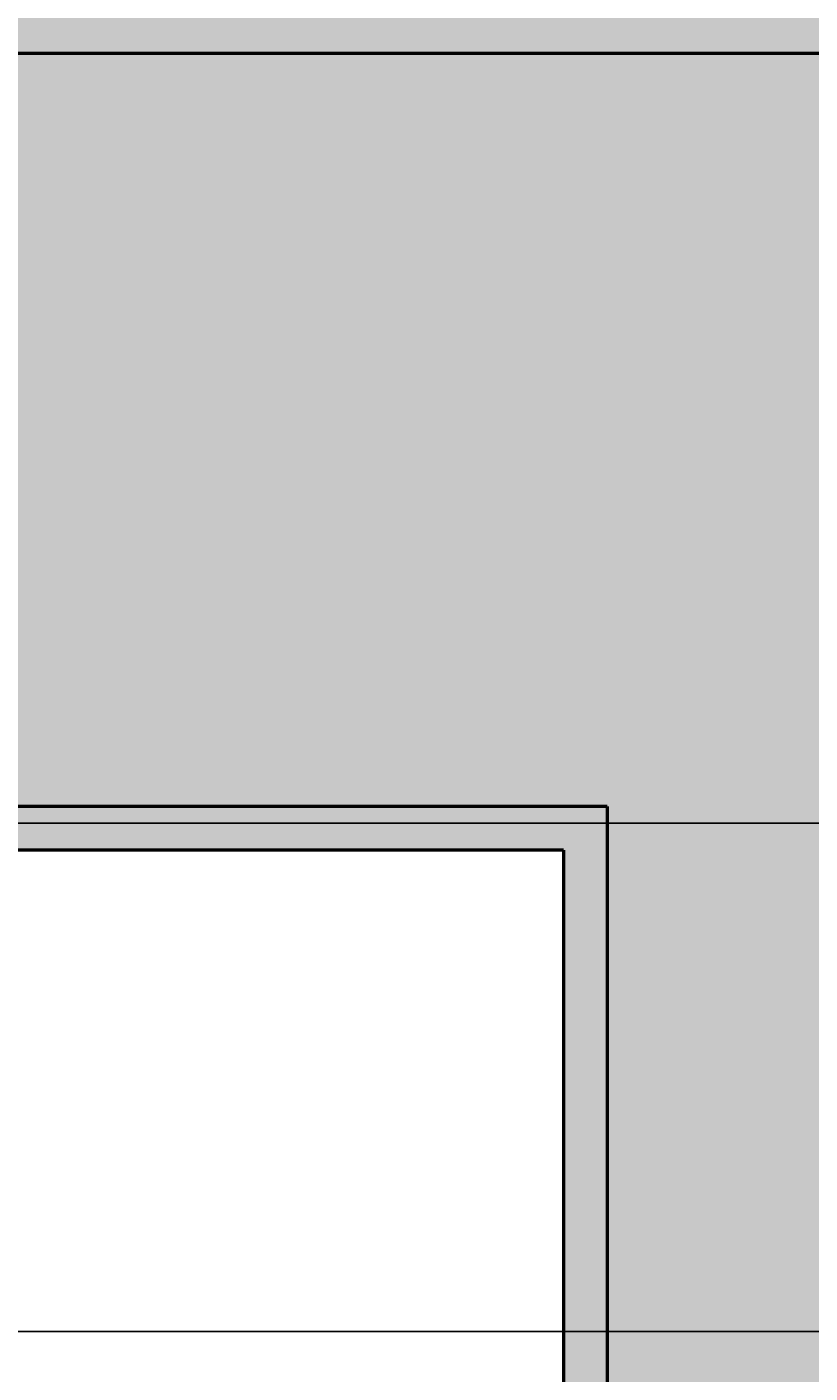
# Model space of a CAD drawing. Units: inches. Extents: x -12 to 334, y -10 to 186.
# Tile 5 of 77: x 24 to 42, y 49 to 79. Entities that reach past the tile are written whole.
import ezdxf

# ---------------------------------------------------------------- set-up
doc = ezdxf.new("R2010")
doc.units = ezdxf.units.IN
doc.header["$MEASUREMENT"] = 0
for name, color, linetype, lineweight in [('M-DIMS', 2, 'Continuous', 18), ('M-EQPM', 7, 'Continuous', 50), ('M-EQPM-PATT', 8, 'Continuous', 18)]:
    doc.layers.add(name, color=color, linetype=linetype, lineweight=lineweight)
doc.styles.get("Standard").update_dxf_attribs({"font": 'arial.ttf'})
doc.dimstyles.get("Standard").update_dxf_attribs({"dimtxt": 0.18, "dimasz": 0.18, "dimexe": 0.18, "dimexo": 0.0625, "dimgap": 0.09, "dimtad": 0, "dimtih": 1, "dimtoh": 1, "dimdec": 4, "dimzin": 0, "dimdsep": 46, "dimtxsty": 'Standard', "dimcen": 0.09, "dimadec": 0, "dimazin": 0, "dimtfac": 1, "dimtdec": 4, "dimtofl": 0, "dimtmove": 0, "dimatfit": 3, "dimfxl": 1, "dimtolj": 1, "dimtzin": 0, "dimarcsym": 0})

# ---------------------------------------------------------------- blocks, each defined once
blk = doc.blocks.new('*D1')
at = {"layer": 'Defpoints', "color": 0, "transparency": 16777216}
for p in [(281.426, 91.899), (3.376, 80.692), (281.426, 14.304)]:
    blk.add_point(p, dxfattribs=at)
at = {"layer": 'M-DIMS', "color": 0, "lineweight": -2, "transparency": 16777216}
for p, q in [((281.426, 91.836), (281.426, 14.124)), ((3.376, 80.629), (3.376, 14.124)), ((3.556, 14.304), (141.935, 14.304)), ((281.246, 14.304), (142.867, 14.304))]:
    blk.add_line(p, q, dxfattribs=at)
at = {"layer": 'M-DIMS', "color": 0, "transparency": 16777216}
for points in [[(3.556, 14.334), (3.556, 14.274), (3.376, 14.304)], [(281.246, 14.334), (281.246, 14.274), (281.426, 14.304)]]:
    blk.add_solid(points, dxfattribs=at)
at = {"layer": 'M-DIMS', "color": 0, "transparency": 16777216, "insert": (142.401, 14.304), "char_height": 0.18, "attachment_point": 5}
blk.add_mtext('\\A1;278.05', dxfattribs=at)
blk = doc.blocks.new('*D6')
at = {"layer": 'Defpoints', "color": 0, "transparency": 16777216}
for p in [(-11.174, 60.487), (23.581, 60.487), (32.1, 33.675)]:
    blk.add_point(p, dxfattribs=at)
at = {"layer": 'M-DIMS', "color": 0, "lineweight": -2, "transparency": 16777216}
for p, q in [((23.518, 60.487), (-11.354, 60.487)), ((-11.174, 60.307), (-11.174, 47.263)), ((-11.174, 33.855), (-11.174, 46.899)), ((32.038, 33.675), (-11.354, 33.675))]:
    blk.add_line(p, q, dxfattribs=at)
at = {"layer": 'M-DIMS', "color": 0, "transparency": 16777216}
for points in [[(-11.204, 60.307), (-11.144, 60.307), (-11.174, 60.487)], [(-11.204, 33.855), (-11.144, 33.855), (-11.174, 33.675)]]:
    blk.add_solid(points, dxfattribs=at)
at = {"layer": 'M-DIMS', "color": 0, "transparency": 16777216, "insert": (-11.174, 47.081), "char_height": 0.18, "attachment_point": 5}
blk.add_mtext('\\A1;26.81', dxfattribs=at)
blk = doc.blocks.new('*D14')
at = {"layer": 'Defpoints', "color": 0, "transparency": 16777216}
for p in [(63.5, 109.058), (-11.174, 49.45), (64.207, 49.45)]:
    blk.add_point(p, dxfattribs=at)
at = {"layer": 'M-DIMS', "color": 0, "lineweight": -2, "transparency": 16777216}
for p, q in [((63.438, 109.058), (-11.354, 109.058)), ((-11.174, 108.878), (-11.174, 79.436)), ((-11.174, 49.63), (-11.174, 79.072)), ((64.144, 49.45), (-11.354, 49.45))]:
    blk.add_line(p, q, dxfattribs=at)
at = {"layer": 'M-DIMS', "color": 0, "transparency": 16777216}
for points in [[(-11.204, 108.878), (-11.144, 108.878), (-11.174, 109.058)], [(-11.204, 49.63), (-11.144, 49.63), (-11.174, 49.45)]]:
    blk.add_solid(points, dxfattribs=at)
at = {"layer": 'M-DIMS', "color": 0, "transparency": 16777216, "insert": (-11.174, 79.254), "char_height": 0.18, "attachment_point": 5}
blk.add_mtext('\\A1;59.61', dxfattribs=at)
blk = doc.blocks.new('*D35')
at = {"layer": 'Defpoints', "color": 0, "transparency": 16777216}
for p in [(216.428, 98.108), (-11.174, 61.105), (216.428, 61.105)]:
    blk.add_point(p, dxfattribs=at)
at = {"layer": 'M-DIMS', "color": 0, "lineweight": -2, "transparency": 16777216}
for p, q in [((216.365, 98.108), (-11.354, 98.108)), ((-11.174, 97.928), (-11.174, 79.788)), ((-11.174, 61.285), (-11.174, 79.424)), ((216.365, 61.105), (-11.354, 61.105))]:
    blk.add_line(p, q, dxfattribs=at)
at = {"layer": 'M-DIMS', "color": 0, "transparency": 16777216}
for points in [[(-11.204, 97.928), (-11.144, 97.928), (-11.174, 98.108)], [(-11.204, 61.285), (-11.144, 61.285), (-11.174, 61.105)]]:
    blk.add_solid(points, dxfattribs=at)
at = {"layer": 'M-DIMS', "color": 0, "transparency": 16777216, "insert": (-11.174, 79.606), "char_height": 0.18, "attachment_point": 5}
blk.add_mtext('\\A1;37', dxfattribs=at)
blk = doc.blocks.new('*D39')
at = {"layer": 'Defpoints', "color": 0, "transparency": 16777216}
for p in [(279.726, 80.692), (-11.174, 45.854), (269.381, 45.854)]:
    blk.add_point(p, dxfattribs=at)
at = {"layer": 'M-DIMS', "color": 0, "lineweight": -2, "transparency": 16777216}
for p, q in [((279.664, 80.692), (-11.354, 80.692)), ((-11.174, 80.512), (-11.174, 63.455)), ((-11.174, 46.034), (-11.174, 63.091)), ((269.318, 45.854), (-11.354, 45.854))]:
    blk.add_line(p, q, dxfattribs=at)
at = {"layer": 'M-DIMS', "color": 0, "transparency": 16777216}
for points in [[(-11.204, 80.512), (-11.144, 80.512), (-11.174, 80.692)], [(-11.204, 46.034), (-11.144, 46.034), (-11.174, 45.854)]]:
    blk.add_solid(points, dxfattribs=at)
at = {"layer": 'M-DIMS', "color": 0, "transparency": 16777216, "insert": (-11.174, 63.273), "char_height": 0.18, "attachment_point": 5}
blk.add_mtext('\\A1;34.84', dxfattribs=at)

msp = doc.modelspace()

# ---------------------------------------------------------------- hatches: boundary and pattern name
at = {"layer": 'M-EQPM-PATT'}
h = msp.add_hatch(color=256, dxfattribs=at)
h.set_gradient(color1=(99, 100, 102), color2=(99, 100, 102), tint=1)
h.paths.add_polyline_path([(4.3766, 80.754, -0.4132606), (23.5807, 99.8958), (37.1002, 99.8958), (37.1002, 127.7078), (32.1002, 127.7078), (32.1002, 125.2078), (36.1002, 125.2078), (36.1002, 100.8958), (23.5807, 100.8958, 1), (23.5807, 60.4872), (36.1002, 60.4872), (36.1002, 36.1752), (32.1002, 36.1752), (32.1002, 33.6752), (37.1002, 33.6752), (37.1002, 61.4872), (23.5807, 61.4872, -0.384914), (4.4744, 78.754), (72.9244, 78.754), (72.9244, 69.6117), (75.9244, 69.6117), (75.9244, 89.8963), (72.9244, 89.8963), (72.9244, 80.754)])
h.paths.add_polyline_path([(54.1002, 125.2078), (58.1002, 125.2078), (58.1002, 127.7078), (53.1002, 127.7078), (53.1002, 99.8958), (64.5, 99.8958), (64.5, 109.0583), (63.5, 109.0583), (63.5, 100.8958), (54.1002, 100.8958)], flags=17)
h.paths.add_polyline_path([(53.1002, 33.6752), (58.1002, 33.6752), (58.1002, 36.1752), (54.1002, 36.1752), (54.1002, 60.4872), (64.2068, 60.4872), (64.2068, 49.4497), (87.8879, 49.4497), (87.8879, 55.3205), (104.8919, 55.3205), (104.8919, 30.8541), (99.8919, 30.8541), (99.8919, 28.8541), (105.8919, 28.8541), (105.8919, 56.3205), (87.8879, 56.3205), (87.8879, 63.6117), (86.8879, 63.6117), (86.8879, 50.4497), (65.0061, 50.4497), (65.0061, 63.6117), (64.5, 63.6117), (64.5, 61.4872), (53.1002, 61.4872)])
h.paths.add_polyline_path([(121.8919, 28.8541), (121.8919, 30.8541), (116.8919, 30.8541), (116.8919, 45.8541), (209.6965, 45.8541), (209.9204, 46.8541), (115.8919, 46.8541), (115.8919, 28.8541)])
h.paths.add_polyline_path([(221.5761, 32.8541), (216.5761, 32.8541), (216.5761, 30.8541), (222.5761, 30.8541), (222.5761, 46.8541), (209.9204, 46.8541), (209.6965, 45.8541), (221.5761, 45.8541)])
h.paths.add_polyline_path([(233.5761, 45.8541), (249.8485, 45.8541), (249.3759, 46.8541), (232.5761, 46.8541), (232.5761, 30.8541), (238.5761, 30.8541), (238.5761, 32.8541), (233.5761, 32.8541)])
h = msp.add_hatch(color=256, dxfattribs=at)
h.set_gradient(color1=(205, 32, 39), color2=(205, 32, 39), tint=1)
h.paths.add_polyline_path([(64.5, 80.754), (64.5, 89.8963), (226.6083, 89.8963, -1), (226.6083, 69.6117), (64.5, 69.6117), (64.5, 78.754), (4.4744, 78.754, 0.384914), (23.5807, 61.4872), (37.1002, 61.4872), (37.1002, 33.6752), (53.1002, 33.6752), (53.1002, 61.4872), (64.5, 61.4872), (64.5, 63.6117), (226.6083, 63.6117, 1), (226.6083, 95.8963), (64.5, 95.8963), (64.5, 99.8958), (53.1002, 99.8958), (53.1002, 127.7078), (37.1002, 127.7078), (37.1002, 99.8958), (23.5807, 99.8958, 0.4132606), (4.3766, 80.754)])
h.paths.add_polyline_path([(64.5, 91.8963), (64.5, 93.8963), (226.6083, 93.8963, -1), (226.6083, 65.6117), (64.5, 65.6117), (64.5, 67.6117), (226.6083, 67.6117, 1), (226.6083, 91.8963)], flags=16)

# ---------------------------------------------------------------- linework, layer by layer
at = {"layer": 'M-EQPM'}
for p, q in [((72.9244, 78.754), (4.4744, 78.754)), ((37.1002, 61.4872), (37.1002, 33.6752)), ((36.1002, 60.4872), (36.1002, 36.1752))]:
    msp.add_line(p, q, dxfattribs=at)
for points in [[(36.1002, 60.4872), (23.5807, 60.4872, -1), (23.5807, 100.8958), (36.1002, 100.8958)], [(37.1002, 61.4872), (23.5807, 61.4872, -0.384914), (4.4744, 78.754, -0.384914)]]:
    msp.add_lwpolyline(points, format="xyb", dxfattribs=at)

# ---------------------------------------------------------------- dimensions: what is measured, and where the dimension line sits
at = {"layer": 'M-DIMS'}
for base, p1, p2, override, picture, middle in [((-11.1736, 49.4497), (63.5, 109.0583), (64.2068, 49.4497), {"dimdec": 2, "dimlfac": 1, "dimrnd": 0, "dimzin": 0, "dimdsep": 46, "dimlunit": 2}, '*D14', (-11.1735, 79.254)), ((-11.1736, 61.1045), (216.4278, 98.1081), (216.4278, 61.1045), {"dimdec": 0, "dimlfac": 1, "dimrnd": 0, "dimzin": 0, "dimdsep": 46, "dimlunit": 2}, '*D35', (-11.1735, 79.6063)), ((-11.1736, 45.8541), (279.7263, 80.6915), (269.3808, 45.8541), {"dimdec": 2, "dimlfac": 1, "dimrnd": 0, "dimzin": 0, "dimdsep": 46, "dimlunit": 2}, '*D39', (-11.1735, 63.2728)), ((-11.1736, 60.4872), (32.1002, 33.6752), (23.5807, 60.4872), {"dimdec": 2, "dimlfac": 1, "dimrnd": 0, "dimzin": 0, "dimdsep": 46, "dimlunit": 2}, '*D6', (-11.1735, 47.0812))]:
    dim = msp.add_linear_dim(base=base, p1=p1, p2=p2, angle=90, dimstyle='Standard', override=override, dxfattribs=at)
    dim.commit()
    dim.dimension.update_dxf_attribs({"geometry": picture, "text_midpoint": middle})
dim = msp.add_linear_dim(base=(281.4256, 14.3041), p1=(3.3765, 80.6915), p2=(281.4256, 91.8988), dimstyle='Standard', override={"dimdec": 2, "dimlfac": 1, "dimrnd": 0, "dimzin": 0, "dimdsep": 46, "dimlunit": 2}, dxfattribs=at)
dim.commit()
dim.dimension.update_dxf_attribs({"geometry": '*D1', "text_midpoint": (142.401, 14.3041)})

doc.saveas('drawing.dxf')
